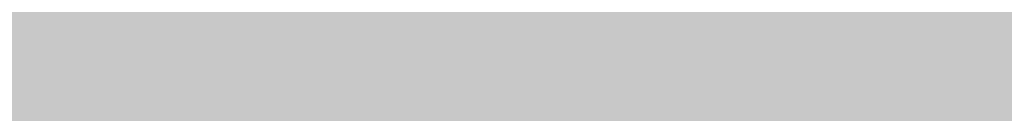
# Model space of a CAD drawing. Units: millimetres. Extents: x 0 to 2267, y 0 to 1823.
# Tile 52 of 256: x 1596.855 to 1600.369, y 1226.386 to 1226.718. Entities that reach past the tile are written whole.
import ezdxf

# ---------------------------------------------------------------- set-up
doc = ezdxf.new("R2010")
doc.units = ezdxf.units.MM
doc.header["$MEASUREMENT"] = 0
doc.layers.add('M-HATC', color=252, linetype='Continuous', lineweight=18)

msp = doc.modelspace()

# ---------------------------------------------------------------- hatches: boundary and pattern name
at = {"layer": 'M-HATC'}
h = msp.add_hatch(color=256, dxfattribs=at)
h.dxf.hatch_style = 1
h.paths.add_polyline_path([(2055.771, 1603.062), (1381.0868, 1603.062), (1381.0868, 1598.062), (2055.771, 1598.062)])
h.paths.add_polyline_path([(2055.771, 1598.062), (1381.0868, 1598.062), (1381.0868, 1593.062), (2055.771, 1593.062)])
h.paths.add_polyline_path([(2051.3074, 1536.7609), (1385.5504, 1536.7609), (1385.5504, 1526.7609), (1387.5504, 1526.7609), (1388.5366, 1525.0528), (1385.3319, 1521.2335), (1385.3319, 1521.2226), (2050.2542, 1522.7491), (2048.3212, 1525.0528), (2049.3074, 1526.7609), (2051.3074, 1526.7609)])
edge = h.paths.add_edge_path()
edge.add_arc((1847.5345, 1379.1492), 135, 222.603061, 222.890851, ccw=False)
edge.add_line((1748.1663, 1287.7656), (1683.0921, 1287.7656))
edge.add_arc((1583.7239, 1379.1492), 135, 317.109149, 317.396939, ccw=False)
edge.add_arc((1678.9686, 1290.6707), 5, 222.8909, 317.1091, ccw=False)
edge.add_arc((1774.2133, 1379.1492), 135, 222.603061, 222.890851, ccw=False)
edge.add_line((1674.8451, 1287.7656), (1609.7709, 1287.7656))
edge.add_arc((1510.4027, 1379.1492), 135, 317.109149, 317.396939, ccw=False)
edge.add_arc((1605.6474, 1290.6707), 5, 222.8909, 317.1091, ccw=False)
edge.add_arc((1700.8921, 1379.1492), 135, 222.603061, 222.890851, ccw=False)
edge.add_line((1601.5239, 1287.7656), (1536.4497, 1287.7656))
edge.add_arc((1437.0815, 1379.1492), 135, 317.109149, 317.396939, ccw=False)
edge.add_arc((1532.3262, 1290.6707), 5, 222.8909, 317.1091, ccw=False)
edge.add_arc((1627.5709, 1379.1492), 135, 222.603061, 222.890851, ccw=False)
edge.add_line((1528.2027, 1287.7656), (1505.9289, 1287.7656))
edge.add_spline(control_points=[(1505.9289, 1287.7656), (1504.2622, 1287.7656), (1504.2622, 1282.7656), (1505.9289, 1282.7656)], knot_values=[0, 0, 0, 0, 5, 5, 5, 5], degree=3, periodic=0)
edge.add_line((1505.9289, 1282.7656), (1930.9289, 1282.7656))
edge.add_spline(control_points=[(1930.9289, 1282.7656), (1932.5956, 1282.7656), (1932.5956, 1287.7656), (1930.9289, 1287.7656)], knot_values=[0, 0, 0, 0, 5, 5, 5, 5], degree=3, periodic=0)
edge.add_line((1930.9289, 1287.7656), (1903.0557, 1287.7656))
edge.add_arc((1803.6875, 1379.1492), 135, 317.109149, 317.396939, ccw=False)
edge.add_arc((1898.9322, 1290.6707), 5, 222.8909, 317.1091, ccw=False)
edge.add_arc((1994.1769, 1379.1492), 135, 222.603061, 222.890851, ccw=False)
edge.add_line((1894.8087, 1287.7656), (1829.7345, 1287.7656))
edge.add_arc((1730.3663, 1379.1492), 135, 317.109149, 317.396939, ccw=False)
edge.add_arc((1825.611, 1290.6707), 5, 222.8909, 317.1091, ccw=False)
edge.add_arc((1920.8557, 1379.1492), 135, 222.603061, 222.890851, ccw=False)
edge.add_line((1821.4875, 1287.7656), (1756.4133, 1287.7656))
edge.add_arc((1657.0451, 1379.1492), 135, 317.109149, 317.396939, ccw=False)
edge.add_arc((1752.2898, 1290.6707), 5, 222.8909, 317.1091, ccw=False)
edge = h.paths.add_edge_path()
edge.add_spline(control_points=[(1843.4289, 1227.2475), (1845.0956, 1227.2475), (1845.0956, 1232.2475), (1843.4289, 1232.2475)], knot_values=[0, 0, 0, 0, 5, 5, 5, 5], degree=3, periodic=0)
edge.add_line((1843.4289, 1232.2475), (1593.4289, 1232.2475))
edge.add_spline(control_points=[(1593.4289, 1232.2475), (1591.7622, 1232.2475), (1591.7622, 1227.2475), (1593.4289, 1227.2475)], knot_values=[0, 0, 0, 0, 5, 5, 5, 5], degree=3, periodic=0)
edge.add_line((1593.4289, 1227.2475), (1843.4289, 1227.2475))
h.paths.add_polyline_path([(1905.9289, 1127.4171), (1530.9289, 1127.4171, 0.414214), (1520.9289, 1117.4171), (1530.9289, 1117.4171), (1915.9289, 1117.4171, 0.414214)])
edge = h.paths.add_edge_path()
edge.add_arc((1397.0858, 1498.4078), 12.7299, 90.78215, 190.87871, ccw=False)
edge.add_line((1396.912, 1511.1365), (1428.0097, 1511.3488))
edge.add_line((1428.0097, 1511.3488), (1433.0097, 1511.3488))
edge.add_line((1433.0097, 1511.3488), (1434.439, 1511.3488))
edge.add_arc((1419.474, 1498.0804), 20, 41.561, 74.08211)
edge.add_line((1424.9592, 1517.3135), (1399.9351, 1517.2561))
edge.add_spline(control_points=[(1399.9307, 1517.2561), (1399.884, 1517.2131), (1399.8328, 1517.1689), (1399.7774, 1517.1236)], knot_values=[11.567499, 11.567499, 11.567499, 11.567499, 11.814249, 11.814249, 11.814249, 11.814249], degree=3, periodic=0)
edge.add_spline(control_points=[(1399.6328, 1517.0099), (1399.5831, 1516.9721), (1399.5307, 1516.9338), (1399.4759, 1516.8947)], knot_values=[11.167718, 11.167718, 11.167718, 11.167718, 11.365188, 11.365188, 11.365188, 11.365188], degree=3, periodic=0)
edge.add_spline(control_points=[(1399.3398, 1516.8001), (1399.1514, 1516.6719), (1398.9384, 1516.5377), (1398.704, 1516.3994)], knot_values=[10.376405, 10.376405, 10.376405, 10.376405, 11.00994, 11.00994, 11.00994, 11.00994], degree=3, periodic=0)
edge.add_spline(control_points=[(1398.6572, 1516.3719), (1398.5789, 1516.326), (1398.4983, 1516.2797), (1398.4155, 1516.2331)], knot_values=[10.125175, 10.125175, 10.125175, 10.125175, 10.334406, 10.334406, 10.334406, 10.334406], degree=3, periodic=0)
edge.add_spline(control_points=[(1398.2642, 1516.1487), (1398.196, 1516.1111), (1398.1263, 1516.0732), (1398.0555, 1516.0351)], knot_values=[9.832246, 9.832246, 9.832246, 9.832246, 9.999658, 9.999658, 9.999658, 9.999658], degree=3, periodic=0)
edge.add_spline(control_points=[(1397.9987, 1516.0048), (1397.7312, 1515.8621), (1397.446, 1515.7171), (1397.1466, 1515.5714)], knot_values=[9.161808, 9.161808, 9.161808, 9.161808, 9.787769, 9.787769, 9.787769, 9.787769], degree=3, periodic=0)
edge.add_spline(control_points=[(1397.1466, 1515.5714), (1396.8418, 1515.423), (1396.5222, 1515.274), (1396.1914, 1515.1262)], knot_values=[8.524455, 8.524455, 8.524455, 8.524455, 9.161808, 9.161808, 9.161808, 9.161808], degree=3, periodic=0)
edge.add_spline(control_points=[(1396.0777, 1515.0756), (1395.9854, 1515.0348), (1395.8922, 1514.994), (1395.7983, 1514.9534)], knot_values=[8.275193, 8.275193, 8.275193, 8.275193, 8.451726, 8.451726, 8.451726, 8.451726], degree=3, periodic=0)
edge.add_spline(control_points=[(1395.6018, 1514.8691), (1395.4997, 1514.8257), (1395.3968, 1514.7824), (1395.2932, 1514.7394)], knot_values=[7.962917, 7.962917, 7.962917, 7.962917, 8.152764, 8.152764, 8.152764, 8.152764], degree=3, periodic=0)
edge.add_spline(control_points=[(1395.2116, 1514.7057), (1394.8278, 1514.5475), (1394.4345, 1514.3929), (1394.0364, 1514.2442)], knot_values=[7.21254, 7.21254, 7.21254, 7.21254, 7.913148, 7.913148, 7.913148, 7.913148], degree=3, periodic=0)
edge.add_spline(control_points=[(1394.0364, 1514.2442), (1393.7076, 1514.1214), (1393.3754, 1514.0027), (1393.0427, 1513.8895)], knot_values=[6.633733, 6.633733, 6.633733, 6.633733, 7.21254, 7.21254, 7.21254, 7.21254], degree=3, periodic=0)
edge.add_spline(control_points=[(1392.8214, 1513.815), (1392.7198, 1513.7812), (1392.6181, 1513.7479), (1392.5166, 1513.7152)], knot_values=[6.328796, 6.328796, 6.328796, 6.328796, 6.505493, 6.505493, 6.505493, 6.505493], degree=3, periodic=0)
edge.add_spline(control_points=[(1392.5166, 1513.7152), (1392.3187, 1513.6515), (1392.1212, 1513.59), (1391.9244, 1513.531)], knot_values=[5.984605, 5.984605, 5.984605, 5.984605, 6.328796, 6.328796, 6.328796, 6.328796], degree=3, periodic=0)
edge.add_spline(control_points=[(1391.7915, 1513.4915), (1391.3122, 1513.3501), (1390.8384, 1513.2239), (1390.3784, 1513.1171)], knot_values=[5.066697, 5.066697, 5.066697, 5.066697, 5.907055, 5.907055, 5.907055, 5.907055], degree=3, periodic=0)
edge.add_spline(control_points=[(1390.3784, 1513.1171), (1390.1797, 1513.071), (1389.9836, 1513.0284), (1389.7907, 1512.9899)], knot_values=[4.70367, 4.70367, 4.70367, 4.70367, 5.066695, 5.066695, 5.066695, 5.066695], degree=3, periodic=0)
edge.add_spline(control_points=[(1389.422, 1512.9204), (1389.2459, 1512.8892), (1389.0729, 1512.8617), (1388.9036, 1512.8381)], knot_values=[4.130571, 4.130571, 4.130571, 4.130571, 4.469816, 4.469816, 4.469816, 4.469816], degree=3, periodic=0)
edge.add_spline(control_points=[(1388.9036, 1512.8381), (1388.591, 1512.7946), (1388.2911, 1512.7644), (1388.0071, 1512.7494)], knot_values=[3.504031, 3.504031, 3.504031, 3.504031, 4.130571, 4.130571, 4.130571, 4.130571], degree=3, periodic=0)
edge.add_spline(control_points=[(1387.9356, 1512.7459), (1387.8538, 1512.7423), (1387.7733, 1512.74), (1387.6944, 1512.739)], knot_values=[3.268866, 3.268866, 3.268866, 3.268866, 3.451164, 3.451164, 3.451164, 3.451164], degree=3, periodic=0)
edge.add_spline(control_points=[(1387.3351, 1512.7443), (1387.2076, 1512.7499), (1387.0847, 1512.7597), (1386.967, 1512.7739)], knot_values=[2.670686, 2.670686, 2.670686, 2.670686, 2.984, 2.984, 2.984, 2.984], degree=3, periodic=0)
edge.add_spline(control_points=[(1386.8327, 1512.7922), (1386.8209, 1512.7941), (1386.8092, 1512.7959), (1386.7975, 1512.7979)], knot_values=[2.516981, 2.516981, 2.516981, 2.516981, 2.549528, 2.549528, 2.549528, 2.549528], degree=3, periodic=0)
edge.add_spline(control_points=[(1386.4526, 1512.8735), (1386.4257, 1512.881), (1386.3993, 1512.889), (1386.3733, 1512.8972)], knot_values=[2.095869, 2.095869, 2.095869, 2.095869, 2.17941, 2.17941, 2.17941, 2.17941], degree=3, periodic=0)
edge.add_spline(control_points=[(1386.0691, 1513.0189), (1386.0634, 1513.0217), (1386.0577, 1513.0246), (1386.052, 1513.0275)], knot_values=[1.72453, 1.72453, 1.72453, 1.72453, 1.745933, 1.745933, 1.745933, 1.745933], degree=3, periodic=0)
edge.add_arc((1399.474, 1498.0804), 20, 131.82432, 180)
edge.add_arc((1630.3336, 1505.5484), 250.9708, 181.705176, 236.427975)
edge.add_arc((1605.3399, 1483.3044), 218.7822, 238.660829, 243.34961)
edge.add_arc((1647.0911, 1510.3592), 262.8986, 183.129836, 237.853442, ccw=False)
h.paths.add_polyline_path([(1406.5369, 1391.9644, 0.149382), (1491.5506, 1296.4418, -0.129517)], flags=17)
edge = h.paths.add_edge_path()
edge.add_arc((2037.3838, 1498.0804), 20, 0, 48.26587)
edge.add_spline(control_points=[(2050.6973, 1513.0052), (2050.6512, 1512.9847), (2050.6034, 1512.9655), (2050.5539, 1512.9477)], knot_values=[1.835652, 1.835652, 1.835652, 1.835652, 2.000781, 2.000781, 2.000781, 2.000781], degree=3, periodic=0)
edge.add_spline(control_points=[(2050.4616, 1512.9166), (2050.479, 1512.9221), (2050.4963, 1512.9277), (2050.5133, 1512.9335)], knot_values=[2.045477, 2.045477, 2.045477, 2.045477, 2.101389, 2.101389, 2.101389, 2.101389], degree=3, periodic=0)
edge.add_spline(control_points=[(2050.129, 1512.8342), (2050.1984, 1512.8473), (2050.2657, 1512.8623), (2050.3308, 1512.8792)], knot_values=[2.237629, 2.237629, 2.237629, 2.237629, 2.435841, 2.435841, 2.435841, 2.435841], degree=3, periodic=0)
edge.add_spline(control_points=[(2050.0946, 1512.8278), (2050.1061, 1512.8299), (2050.1176, 1512.832), (2050.129, 1512.8342)], knot_values=[2.435841, 2.435841, 2.435841, 2.435841, 2.468321, 2.468321, 2.468321, 2.468321], degree=3, periodic=0)
edge.add_spline(control_points=[(2049.7843, 1512.7851), (2049.8552, 1512.7922), (2049.9243, 1512.8008), (2049.9917, 1512.8109)], knot_values=[2.563852, 2.563852, 2.563852, 2.563852, 2.748541, 2.748541, 2.748541, 2.748541], degree=3, periodic=0)
edge.add_spline(control_points=[(2049.4052, 1512.7617), (2049.5364, 1512.7653), (2049.6629, 1512.773), (2049.7843, 1512.7851)], knot_values=[2.748541, 2.748541, 2.748541, 2.748541, 3.064882, 3.064882, 3.064882, 3.064882], degree=3, periodic=0)
edge.add_spline(control_points=[(2049.1698, 1512.7597), (2049.2336, 1512.7591), (2049.2965, 1512.7594), (2049.3584, 1512.7606)], knot_values=[3.102309, 3.102309, 3.102309, 3.102309, 3.2503, 3.2503, 3.2503, 3.2503], degree=3, periodic=0)
edge.add_spline(control_points=[(2048.8573, 1512.7691), (2048.9638, 1512.7638), (2049.068, 1512.7606), (2049.1698, 1512.7597)], knot_values=[3.2503, 3.2503, 3.2503, 3.2503, 3.486069, 3.486069, 3.486069, 3.486069], degree=3, periodic=0)
edge.add_spline(control_points=[(2048.6924, 1512.7789), (2048.3729, 1512.8009), (2048.0345, 1512.8411), (2047.6817, 1512.897)], knot_values=[3.606429, 3.606429, 3.606429, 3.606429, 4.2989, 4.2989, 4.2989, 4.2989], degree=3, periodic=0)
edge.add_spline(control_points=[(2047.6817, 1512.897), (2047.5458, 1512.9185), (2047.4077, 1512.9424), (2047.2678, 1512.9685)], knot_values=[4.2989, 4.2989, 4.2989, 4.2989, 4.565769, 4.565769, 4.565769, 4.565769], degree=3, periodic=0)
edge.add_spline(control_points=[(2047.2678, 1512.9685), (2047.1449, 1512.9914), (2047.0207, 1513.016), (2046.8951, 1513.0422)], knot_values=[4.565769, 4.565769, 4.565769, 4.565769, 4.799971, 4.799971, 4.799971, 4.799971], degree=3, periodic=0)
edge.add_spline(control_points=[(2046.8951, 1513.0422), (2046.5286, 1513.1188), (2046.1513, 1513.209), (2045.7676, 1513.3107)], knot_values=[4.799971, 4.799971, 4.799971, 4.799971, 5.483718, 5.483718, 5.483718, 5.483718], degree=3, periodic=0)
edge.add_spline(control_points=[(2045.7676, 1513.3107), (2045.3724, 1513.4154), (2044.9704, 1513.5322), (2044.5662, 1513.6588)], knot_values=[5.483718, 5.483718, 5.483718, 5.483718, 6.187866, 6.187866, 6.187866, 6.187866], degree=3, periodic=0)
edge.add_spline(control_points=[(2044.5662, 1513.6588), (2044.4149, 1513.7061), (2044.2633, 1513.7549), (2044.1116, 1513.8048)], knot_values=[6.187866, 6.187866, 6.187866, 6.187866, 6.451551, 6.451551, 6.451551, 6.451551], degree=3, periodic=0)
edge.add_spline(control_points=[(2044.1116, 1513.8048), (2043.9967, 1513.8427), (2043.8817, 1513.8813), (2043.7668, 1513.9205)], knot_values=[6.451551, 6.451551, 6.451551, 6.451551, 6.651434, 6.651434, 6.651434, 6.651434], degree=3, periodic=0)
edge.add_spline(control_points=[(2043.7668, 1513.9205), (2043.3716, 1514.0554), (2042.9774, 1514.1979), (2042.5886, 1514.3458)], knot_values=[6.651434, 6.651434, 6.651434, 6.651434, 7.338879, 7.338879, 7.338879, 7.338879], degree=3, periodic=0)
edge.add_spline(control_points=[(2042.5886, 1514.3458), (2042.1643, 1514.5071), (2041.7465, 1514.6749), (2041.3409, 1514.846)], knot_values=[7.338879, 7.338879, 7.338879, 7.338879, 8.089209, 8.089209, 8.089209, 8.089209], degree=3, periodic=0)
edge.add_spline(control_points=[(2041.3409, 1514.846), (2041.1028, 1514.9465), (2040.869, 1515.0481), (2040.6405, 1515.1502)], knot_values=[8.089209, 8.089209, 8.089209, 8.089209, 8.529587, 8.529587, 8.529587, 8.529587], degree=3, periodic=0)
edge.add_spline(control_points=[(2040.51, 1515.2089), (2040.0824, 1515.4022), (2039.6747, 1515.5971), (2039.295, 1515.7894)], knot_values=[8.613818, 8.613818, 8.613818, 8.613818, 9.44571, 9.44571, 9.44571, 9.44571], degree=3, periodic=0)
edge.add_spline(control_points=[(2039.295, 1515.7894), (2039.0618, 1515.9075), (2038.8391, 1516.0246), (2038.6288, 1516.1398)], knot_values=[9.44571, 9.44571, 9.44571, 9.44571, 9.956404, 9.956404, 9.956404, 9.956404], degree=3, periodic=0)
edge.add_spline(control_points=[(2038.6288, 1516.1398), (2038.5187, 1516.2001), (2038.4121, 1516.2598), (2038.309, 1516.3189)], knot_values=[9.956404, 9.956404, 9.956404, 9.956404, 10.223542, 10.223542, 10.223542, 10.223542], degree=3, periodic=0)
edge.add_spline(control_points=[(2038.309, 1516.3189), (2038.2138, 1516.3735), (2038.1216, 1516.4276), (2038.0328, 1516.481)], knot_values=[10.223542, 10.223542, 10.223542, 10.223542, 10.47051, 10.47051, 10.47051, 10.47051], degree=3, periodic=0)
edge.add_spline(control_points=[(2038.0328, 1516.481), (2037.7855, 1516.6296), (2037.5639, 1516.773), (2037.3722, 1516.909)], knot_values=[10.47051, 10.47051, 10.47051, 10.47051, 11.15767, 11.15767, 11.15767, 11.15767], degree=3, periodic=0)
edge.add_spline(control_points=[(2037.3722, 1516.909), (2037.2789, 1516.9752), (2037.1927, 1517.0396), (2037.1142, 1517.102)], knot_values=[11.15767, 11.15767, 11.15767, 11.15767, 11.49227, 11.49227, 11.49227, 11.49227], degree=3, periodic=0)
edge.add_spline(control_points=[(2036.8564, 1517.3259), (2036.9148, 1517.2692), (2036.9814, 1517.2103), (2037.0557, 1517.1492)], knot_values=[11.577341, 11.577341, 11.577341, 11.577341, 11.91035, 11.91035, 11.91035, 11.91035], degree=3, periodic=0)
edge.add_spline(control_points=[(2036.8074, 1517.3748), (2036.823, 1517.3587), (2036.8393, 1517.3424), (2036.8564, 1517.3259)], knot_values=[11.91035, 11.91035, 11.91035, 11.91035, 12.007402, 12.007402, 12.007402, 12.007402], degree=3, periodic=0)
edge.add_spline(control_points=[(2036.7017, 1517.494), (2036.7104, 1517.483), (2036.7196, 1517.4719), (2036.7291, 1517.4606)], knot_values=[12.184155, 12.184155, 12.184155, 12.184155, 12.255409, 12.255409, 12.255409, 12.255409], degree=3, periodic=0)
edge.add_spline(control_points=[(2036.6159, 1517.6205), (2036.62, 1517.613), (2036.6243, 1517.6055), (2036.6289, 1517.5979)], knot_values=[12.487913, 12.487913, 12.487913, 12.487913, 12.541035, 12.541035, 12.541035, 12.541035], degree=3, periodic=0)
edge.add_spline(control_points=[(2036.5635, 1517.786), (2036.5637, 1517.7794), (2036.5642, 1517.7726), (2036.565, 1517.7658)], knot_values=[12.911761, 12.911761, 12.911761, 12.911761, 12.968286, 12.968286, 12.968286, 12.968286], degree=3, periodic=0)
edge.add_spline(control_points=[(2036.6166, 1517.9304), (2036.6125, 1517.9259), (2036.6086, 1517.9212), (2036.6049, 1517.9165)], knot_values=[13.382527, 13.382527, 13.382527, 13.382527, 13.433791, 13.433791, 13.433791, 13.433791], degree=3, periodic=0)
edge.add_spline(control_points=[(2036.749, 1518.017), (2036.7361, 1518.0116), (2036.7239, 1518.006), (2036.7124, 1518.0002)], knot_values=[13.726299, 13.726299, 13.726299, 13.726299, 13.809928, 13.809928, 13.809928, 13.809928], degree=3, periodic=0)
edge.add_spline(control_points=[(2036.8604, 1518.0528), (2036.8386, 1518.0474), (2036.8181, 1518.0416), (2036.7988, 1518.0353)], knot_values=[13.910887, 13.910887, 13.910887, 13.910887, 14.02153, 14.02153, 14.02153, 14.02153], degree=3, periodic=0)
edge.add_line((2036.9639, 1518.0804), (2032.3838, 1518.0804))
edge.add_line((2032.3838, 1518.0804), (2027.3838, 1518.0804))
edge.add_line((2027.3838, 1518.0804), (2022.3838, 1518.0804))
edge.add_line((2022.3838, 1518.0804), (2017.3838, 1518.0804))
edge.add_arc((2017.3838, 1498.0804), 20, 90, 138.439)
edge.add_line((2002.4188, 1511.3488), (2003.8481, 1511.3488))
edge.add_line((2003.8481, 1511.3488), (2008.8481, 1511.3488))
edge.add_line((2008.8481, 1511.3488), (2039.772, 1511.1377))
edge.add_arc((2039.772, 1498.4078), 12.7299, -10.87871, 90, ccw=False)
edge.add_arc((1789.7668, 1510.3592), 262.8986, 302.146558, 356.870164, ccw=False)
edge.add_arc((1831.5179, 1483.3044), 218.7822, 296.65039, 301.339171)
edge.add_arc((1806.5242, 1505.5484), 250.9708, 303.572025, 358.294824)
h.paths.add_polyline_path([(2030.321, 1391.9644, -0.129517), (1945.3072, 1296.4418, 0.149382)], flags=17)
edge = h.paths.add_edge_path()
edge.add_spline(control_points=[(2037.2464, 1518.0821), (2037.2898, 1518.081), (2037.3355, 1518.0804), (2037.3838, 1518.0804)], knot_values=[0.000012, 0.000012, 0.000012, 0.000012, 0.144754, 0.144754, 0.144754, 0.144754], degree=3, periodic=0)
edge.add_line((2037.3357, 1518.0804), (2037.0096, 1518.0804))
edge.add_spline(control_points=[(2037.0096, 1518.0804), (2036.9822, 1518.0768), (2036.956, 1518.0727), (2036.9312, 1518.0681)], knot_values=[14.13465, 14.13465, 14.13465, 14.13465, 14.247197, 14.247197, 14.247197, 14.247197], degree=3, periodic=0)
edge.add_spline(control_points=[(2036.9312, 1518.0681), (2036.9276, 1518.0674), (2036.9241, 1518.0667), (2036.9205, 1518.0661)], knot_values=[14.118315, 14.118315, 14.118315, 14.118315, 14.13465, 14.13465, 14.13465, 14.13465], degree=3, periodic=0)
edge.add_spline(control_points=[(2036.9205, 1518.0661), (2036.9118, 1518.0644), (2036.9032, 1518.0626), (2036.8948, 1518.0608)], knot_values=[14.078086, 14.078086, 14.078086, 14.078086, 14.118315, 14.118315, 14.118315, 14.118315], degree=3, periodic=0)
edge.add_spline(control_points=[(2036.8948, 1518.0608), (2036.883, 1518.0583), (2036.8716, 1518.0556), (2036.8604, 1518.0528)], knot_values=[14.02153, 14.02153, 14.02153, 14.02153, 14.078086, 14.078086, 14.078086, 14.078086], degree=3, periodic=0)
edge.add_spline(control_points=[(2036.8604, 1518.0528), (2036.8386, 1518.0474), (2036.8181, 1518.0416), (2036.7988, 1518.0353)], knot_values=[13.910887, 13.910887, 13.910887, 13.910887, 14.02153, 14.02153, 14.02153, 14.02153], degree=3, periodic=0)
edge.add_spline(control_points=[(2036.7988, 1518.0353), (2036.7981, 1518.035), (2036.7974, 1518.0348), (2036.7967, 1518.0346)], knot_values=[13.906906, 13.906906, 13.906906, 13.906906, 13.910887, 13.910887, 13.910887, 13.910887], degree=3, periodic=0)
edge.add_spline(control_points=[(2036.7967, 1518.0346), (2036.7882, 1518.0318), (2036.7799, 1518.0289), (2036.7719, 1518.0259)], knot_values=[13.857826, 13.857826, 13.857826, 13.857826, 13.906906, 13.906906, 13.906906, 13.906906], degree=3, periodic=0)
edge.add_spline(control_points=[(2036.7719, 1518.0259), (2036.764, 1518.023), (2036.7564, 1518.02), (2036.749, 1518.017)], knot_values=[13.809928, 13.809928, 13.809928, 13.809928, 13.857826, 13.857826, 13.857826, 13.857826], degree=3, periodic=0)
edge.add_spline(control_points=[(2036.749, 1518.017), (2036.7361, 1518.0116), (2036.7239, 1518.006), (2036.7124, 1518.0002)], knot_values=[13.726299, 13.726299, 13.726299, 13.726299, 13.809928, 13.809928, 13.809928, 13.809928], degree=3, periodic=0)
edge.add_spline(control_points=[(2036.7124, 1518.0002), (2036.7121, 1518), (2036.7118, 1517.9999), (2036.7115, 1517.9997)], knot_values=[13.723993, 13.723993, 13.723993, 13.723993, 13.726299, 13.726299, 13.726299, 13.726299], degree=3, periodic=0)
edge.add_spline(control_points=[(2036.7115, 1517.9997), (2036.7063, 1517.9971), (2036.7013, 1517.9944), (2036.6965, 1517.9917)], knot_values=[13.686536, 13.686536, 13.686536, 13.686536, 13.723993, 13.723993, 13.723993, 13.723993], degree=3, periodic=0)
edge.add_spline(control_points=[(2036.6965, 1517.9917), (2036.6919, 1517.9891), (2036.6874, 1517.9865), (2036.6831, 1517.9839)], knot_values=[13.651251, 13.651251, 13.651251, 13.651251, 13.686536, 13.686536, 13.686536, 13.686536], degree=3, periodic=0)
edge.add_spline(control_points=[(2036.6831, 1517.9839), (2036.6764, 1517.9798), (2036.67, 1517.9757), (2036.6639, 1517.9714)], knot_values=[13.596804, 13.596804, 13.596804, 13.596804, 13.651251, 13.651251, 13.651251, 13.651251], degree=3, periodic=0)
edge.add_spline(control_points=[(2036.6639, 1517.9714), (2036.6636, 1517.9712), (2036.6633, 1517.9709), (2036.6629, 1517.9707)], knot_values=[13.593956, 13.593956, 13.593956, 13.593956, 13.596804, 13.596804, 13.596804, 13.596804], degree=3, periodic=0)
edge.add_spline(control_points=[(2036.6629, 1517.9707), (2036.6603, 1517.9689), (2036.6577, 1517.967), (2036.6552, 1517.9651)], knot_values=[13.570322, 13.570322, 13.570322, 13.570322, 13.593956, 13.593956, 13.593956, 13.593956], degree=3, periodic=0)
edge.add_spline(control_points=[(2036.6552, 1517.9651), (2036.6525, 1517.9631), (2036.6499, 1517.9611), (2036.6474, 1517.9591)], knot_values=[13.545477, 13.545477, 13.545477, 13.545477, 13.570322, 13.570322, 13.570322, 13.570322], degree=3, periodic=0)
edge.add_spline(control_points=[(2036.6474, 1517.9591), (2036.6472, 1517.9589), (2036.6471, 1517.9588), (2036.6469, 1517.9587)], knot_values=[13.543931, 13.543931, 13.543931, 13.543931, 13.545477, 13.545477, 13.545477, 13.545477], degree=3, periodic=0)
edge.add_spline(control_points=[(2036.6469, 1517.9587), (2036.6412, 1517.9541), (2036.6358, 1517.9494), (2036.6307, 1517.9447)], knot_values=[13.488237, 13.488237, 13.488237, 13.488237, 13.543931, 13.543931, 13.543931, 13.543931], degree=3, periodic=0)
edge.add_spline(control_points=[(2036.6307, 1517.9447), (2036.6282, 1517.9423), (2036.6257, 1517.9399), (2036.6233, 1517.9374)], knot_values=[13.460307, 13.460307, 13.460307, 13.460307, 13.488237, 13.488237, 13.488237, 13.488237], degree=3, periodic=0)
edge.add_spline(control_points=[(2036.6233, 1517.9374), (2036.6215, 1517.9356), (2036.6198, 1517.9338), (2036.6181, 1517.932)], knot_values=[13.439712, 13.439712, 13.439712, 13.439712, 13.460307, 13.460307, 13.460307, 13.460307], degree=3, periodic=0)
edge.add_spline(control_points=[(2036.6181, 1517.932), (2036.6176, 1517.9315), (2036.6171, 1517.9309), (2036.6166, 1517.9304)], knot_values=[13.433791, 13.433791, 13.433791, 13.433791, 13.439712, 13.439712, 13.439712, 13.439712], degree=3, periodic=0)
edge.add_spline(control_points=[(2036.6166, 1517.9304), (2036.6125, 1517.9259), (2036.6086, 1517.9212), (2036.6049, 1517.9165)], knot_values=[13.382527, 13.382527, 13.382527, 13.382527, 13.433791, 13.433791, 13.433791, 13.433791], degree=3, periodic=0)
edge.add_spline(control_points=[(2036.6049, 1517.9165), (2036.6026, 1517.9135), (2036.6004, 1517.9104), (2036.5982, 1517.9074)], knot_values=[13.350017, 13.350017, 13.350017, 13.350017, 13.382527, 13.382527, 13.382527, 13.382527], degree=3, periodic=0)
edge.add_spline(control_points=[(2036.5982, 1517.9074), (2036.5972, 1517.9059), (2036.5962, 1517.9043), (2036.5952, 1517.9028)], knot_values=[13.333922, 13.333922, 13.333922, 13.333922, 13.350017, 13.350017, 13.350017, 13.350017], degree=3, periodic=0)
edge.add_spline(control_points=[(2036.5952, 1517.9028), (2036.5945, 1517.9018), (2036.5939, 1517.9009), (2036.5933, 1517.8999)], knot_values=[13.323828, 13.323828, 13.323828, 13.323828, 13.333922, 13.333922, 13.333922, 13.333922], degree=3, periodic=0)
edge.add_spline(control_points=[(2036.5933, 1517.8999), (2036.5905, 1517.8955), (2036.5879, 1517.8909), (2036.5855, 1517.8864)], knot_values=[13.277545, 13.277545, 13.277545, 13.277545, 13.323828, 13.323828, 13.323828, 13.323828], degree=3, periodic=0)
edge.add_spline(control_points=[(2036.5855, 1517.8864), (2036.5836, 1517.8827), (2036.5817, 1517.8789), (2036.5801, 1517.8751)], knot_values=[13.240119, 13.240119, 13.240119, 13.240119, 13.277545, 13.277545, 13.277545, 13.277545], degree=3, periodic=0)
edge.add_spline(control_points=[(2036.5801, 1517.8751), (2036.5795, 1517.8739), (2036.579, 1517.8727), (2036.5785, 1517.8715)], knot_values=[13.228211, 13.228211, 13.228211, 13.228211, 13.240119, 13.240119, 13.240119, 13.240119], degree=3, periodic=0)
edge.add_spline(control_points=[(2036.5785, 1517.8715), (2036.578, 1517.8702), (2036.5774, 1517.869), (2036.5769, 1517.8677)], knot_values=[13.215717, 13.215717, 13.215717, 13.215717, 13.228211, 13.228211, 13.228211, 13.228211], degree=3, periodic=0)
edge.add_spline(control_points=[(2036.5769, 1517.8677), (2036.5755, 1517.864), (2036.5741, 1517.8603), (2036.5729, 1517.8565)], knot_values=[13.179847, 13.179847, 13.179847, 13.179847, 13.215717, 13.215717, 13.215717, 13.215717], degree=3, periodic=0)
edge.add_spline(control_points=[(2036.5729, 1517.8565), (2036.5713, 1517.8515), (2036.5699, 1517.8464), (2036.5687, 1517.8413)], knot_values=[13.132017, 13.132017, 13.132017, 13.132017, 13.179847, 13.179847, 13.179847, 13.179847], degree=3, periodic=0)
edge.add_spline(control_points=[(2036.5687, 1517.8413), (2036.5684, 1517.8402), (2036.5682, 1517.8392), (2036.568, 1517.8382)], knot_values=[13.122482, 13.122482, 13.122482, 13.122482, 13.132017, 13.132017, 13.132017, 13.132017], degree=3, periodic=0)
edge.add_spline(control_points=[(2036.568, 1517.8382), (2036.5676, 1517.8363), (2036.5672, 1517.8345), (2036.5669, 1517.8327)], knot_values=[13.105592, 13.105592, 13.105592, 13.105592, 13.122482, 13.122482, 13.122482, 13.122482], degree=3, periodic=0)
edge.add_spline(control_points=[(2036.5669, 1517.8327), (2036.5662, 1517.8292), (2036.5657, 1517.8257), (2036.5652, 1517.8222)], knot_values=[13.074063, 13.074063, 13.074063, 13.074063, 13.105592, 13.105592, 13.105592, 13.105592], degree=3, periodic=0)
edge.add_spline(control_points=[(2036.5652, 1517.8222), (2036.5652, 1517.8222), (2036.5652, 1517.8222), (2036.5652, 1517.8222)], knot_values=[13.074043, 13.074043, 13.074043, 13.074043, 13.074063, 13.074063, 13.074063, 13.074063], degree=3, periodic=0)
edge.add_spline(control_points=[(2036.5652, 1517.8222), (2036.5644, 1517.8164), (2036.5639, 1517.8106), (2036.5636, 1517.8046)], knot_values=[13.021884, 13.021884, 13.021884, 13.021884, 13.074043, 13.074043, 13.074043, 13.074043], degree=3, periodic=0)
edge.add_spline(control_points=[(2036.5636, 1517.8046), (2036.5636, 1517.804), (2036.5636, 1517.8034), (2036.5635, 1517.8028)], knot_values=[13.01674, 13.01674, 13.01674, 13.01674, 13.021884, 13.021884, 13.021884, 13.021884], degree=3, periodic=0)
edge.add_spline(control_points=[(2036.5635, 1517.8028), (2036.5634, 1517.8005), (2036.5634, 1517.7982), (2036.5634, 1517.7958)], knot_values=[12.996438, 12.996438, 12.996438, 12.996438, 13.01674, 13.01674, 13.01674, 13.01674], degree=3, periodic=0)
edge.add_spline(control_points=[(2036.5634, 1517.7958), (2036.5633, 1517.7926), (2036.5634, 1517.7893), (2036.5635, 1517.786)], knot_values=[12.968286, 12.968286, 12.968286, 12.968286, 12.996438, 12.996438, 12.996438, 12.996438], degree=3, periodic=0)
edge.add_spline(control_points=[(2036.5635, 1517.786), (2036.5637, 1517.7794), (2036.5642, 1517.7726), (2036.565, 1517.7658)], knot_values=[12.911761, 12.911761, 12.911761, 12.911761, 12.968286, 12.968286, 12.968286, 12.968286], degree=3, periodic=0)
edge.add_spline(control_points=[(2036.565, 1517.7658), (2036.565, 1517.7657), (2036.565, 1517.7656), (2036.565, 1517.7656)], knot_values=[12.911017, 12.911017, 12.911017, 12.911017, 12.911761, 12.911761, 12.911761, 12.911761], degree=3, periodic=0)
edge.add_spline(control_points=[(2036.565, 1517.7656), (2036.5654, 1517.7625), (2036.5658, 1517.7593), (2036.5663, 1517.7562)], knot_values=[12.88528, 12.88528, 12.88528, 12.88528, 12.911017, 12.911017, 12.911017, 12.911017], degree=3, periodic=0)
edge.add_spline(control_points=[(2036.5663, 1517.7562), (2036.5667, 1517.7534), (2036.5672, 1517.7506), (2036.5677, 1517.7478)], knot_values=[12.862519, 12.862519, 12.862519, 12.862519, 12.88528, 12.88528, 12.88528, 12.88528], degree=3, periodic=0)
edge.add_spline(control_points=[(2036.5677, 1517.7478), (2036.5678, 1517.7474), (2036.5679, 1517.7469), (2036.568, 1517.7465)], knot_values=[12.858885, 12.858885, 12.858885, 12.858885, 12.862519, 12.862519, 12.862519, 12.862519], degree=3, periodic=0)
edge.add_spline(control_points=[(2036.568, 1517.7465), (2036.5692, 1517.7399), (2036.5707, 1517.7332), (2036.5724, 1517.7264)], knot_values=[12.8053, 12.8053, 12.8053, 12.8053, 12.858885, 12.858885, 12.858885, 12.858885], degree=3, periodic=0)
edge.add_spline(control_points=[(2036.5724, 1517.7264), (2036.5734, 1517.7226), (2036.5745, 1517.7187), (2036.5756, 1517.7149)], knot_values=[12.775176, 12.775176, 12.775176, 12.775176, 12.8053, 12.8053, 12.8053, 12.8053], degree=3, periodic=0)
edge.add_spline(control_points=[(2036.5756, 1517.7149), (2036.5763, 1517.7125), (2036.577, 1517.7102), (2036.5778, 1517.7078)], knot_values=[12.756759, 12.756759, 12.756759, 12.756759, 12.775176, 12.775176, 12.775176, 12.775176], degree=3, periodic=0)
edge.add_spline(control_points=[(2036.5778, 1517.7078), (2036.5781, 1517.7067), (2036.5784, 1517.7057), (2036.5787, 1517.7047)], knot_values=[12.748742, 12.748742, 12.748742, 12.748742, 12.756759, 12.756759, 12.756759, 12.756759], degree=3, periodic=0)
edge.add_spline(control_points=[(2036.5787, 1517.7047), (2036.5808, 1517.6983), (2036.5831, 1517.6919), (2036.5856, 1517.6854)], knot_values=[12.69959, 12.69959, 12.69959, 12.69959, 12.748742, 12.748742, 12.748742, 12.748742], degree=3, periodic=0)
edge.add_spline(control_points=[(2036.5856, 1517.6854), (2036.5876, 1517.68), (2036.5898, 1517.6746), (2036.5921, 1517.6692)], knot_values=[12.659038, 12.659038, 12.659038, 12.659038, 12.69959, 12.69959, 12.69959, 12.69959], degree=3, periodic=0)
edge.add_spline(control_points=[(2036.5921, 1517.6692), (2036.594, 1517.6648), (2036.5959, 1517.6605), (2036.5979, 1517.6561)], knot_values=[12.626806, 12.626806, 12.626806, 12.626806, 12.659038, 12.659038, 12.659038, 12.659038], degree=3, periodic=0)
edge.add_spline(control_points=[(2036.5979, 1517.6561), (2036.5984, 1517.6551), (2036.5989, 1517.6541), (2036.5993, 1517.6531)], knot_values=[12.619394, 12.619394, 12.619394, 12.619394, 12.626806, 12.626806, 12.626806, 12.626806], degree=3, periodic=0)
edge.add_spline(control_points=[(2036.5993, 1517.6531), (2036.6043, 1517.6424), (2036.6099, 1517.6315), (2036.6159, 1517.6205)], knot_values=[12.541039, 12.541039, 12.541039, 12.541039, 12.619394, 12.619394, 12.619394, 12.619394], degree=3, periodic=0)
edge.add_spline(control_points=[(2036.6159, 1517.6205), (2036.6159, 1517.6205), (2036.6159, 1517.6205), (2036.6159, 1517.6205)], knot_values=[12.541035, 12.541035, 12.541035, 12.541035, 12.541039, 12.541039, 12.541039, 12.541039], degree=3, periodic=0)
edge.add_spline(control_points=[(2036.6159, 1517.6205), (2036.62, 1517.613), (2036.6243, 1517.6055), (2036.6289, 1517.5979)], knot_values=[12.487913, 12.487913, 12.487913, 12.487913, 12.541035, 12.541035, 12.541035, 12.541035], degree=3, periodic=0)
edge.add_spline(control_points=[(2036.6289, 1517.5979), (2036.6326, 1517.5916), (2036.6365, 1517.5853), (2036.6406, 1517.5789)], knot_values=[12.443982, 12.443982, 12.443982, 12.443982, 12.487913, 12.487913, 12.487913, 12.487913], degree=3, periodic=0)
edge.add_spline(control_points=[(2036.6406, 1517.5789), (2036.6414, 1517.5776), (2036.6423, 1517.5763), (2036.6431, 1517.5749)], knot_values=[12.434996, 12.434996, 12.434996, 12.434996, 12.443982, 12.443982, 12.443982, 12.443982], degree=3, periodic=0)
edge.add_spline(control_points=[(2036.6431, 1517.5749), (2036.6531, 1517.5596), (2036.6639, 1517.5439), (2036.6756, 1517.528)], knot_values=[12.329647, 12.329647, 12.329647, 12.329647, 12.434996, 12.434996, 12.434996, 12.434996], degree=3, periodic=0)
edge.add_spline(control_points=[(2036.6756, 1517.528), (2036.6839, 1517.5168), (2036.6925, 1517.5055), (2036.7017, 1517.494)], knot_values=[12.255409, 12.255409, 12.255409, 12.255409, 12.329647, 12.329647, 12.329647, 12.329647], degree=3, periodic=0)
edge.add_spline(control_points=[(2036.7017, 1517.494), (2036.7104, 1517.483), (2036.7196, 1517.4719), (2036.7291, 1517.4606)], knot_values=[12.184155, 12.184155, 12.184155, 12.184155, 12.255409, 12.255409, 12.255409, 12.255409], degree=3, periodic=0)
edge.add_spline(control_points=[(2036.7291, 1517.4606), (2036.7436, 1517.4435), (2036.759, 1517.4262), (2036.7753, 1517.4085)], knot_values=[12.075961, 12.075961, 12.075961, 12.075961, 12.184155, 12.184155, 12.184155, 12.184155], degree=3, periodic=0)
edge.add_spline(control_points=[(2036.7753, 1517.4085), (2036.7763, 1517.4075), (2036.7773, 1517.4064), (2036.7783, 1517.4054)], knot_values=[12.069502, 12.069502, 12.069502, 12.069502, 12.075961, 12.075961, 12.075961, 12.075961], degree=3, periodic=0)
edge.add_spline(control_points=[(2036.7783, 1517.4054), (2036.7877, 1517.3953), (2036.7974, 1517.385), (2036.8074, 1517.3748)], knot_values=[12.007402, 12.007402, 12.007402, 12.007402, 12.069502, 12.069502, 12.069502, 12.069502], degree=3, periodic=0)
edge.add_spline(control_points=[(2036.8074, 1517.3748), (2036.823, 1517.3587), (2036.8393, 1517.3424), (2036.8564, 1517.3259)], knot_values=[11.91035, 11.91035, 11.91035, 11.91035, 12.007402, 12.007402, 12.007402, 12.007402], degree=3, periodic=0)
edge.add_spline(control_points=[(2036.8564, 1517.3259), (2036.9148, 1517.2692), (2036.9814, 1517.2103), (2037.0557, 1517.1492)], knot_values=[11.577341, 11.577341, 11.577341, 11.577341, 11.91035, 11.91035, 11.91035, 11.91035], degree=3, periodic=0)
edge.add_spline(control_points=[(2037.0557, 1517.1492), (2037.0747, 1517.1336), (2037.0942, 1517.1179), (2037.1142, 1517.102)], knot_values=[11.49227, 11.49227, 11.49227, 11.49227, 11.577341, 11.577341, 11.577341, 11.577341], degree=3, periodic=0)
edge.add_spline(control_points=[(2037.1142, 1517.102), (2037.1927, 1517.0396), (2037.2789, 1516.9752), (2037.3722, 1516.909)], knot_values=[11.15767, 11.15767, 11.15767, 11.15767, 11.49227, 11.49227, 11.49227, 11.49227], degree=3, periodic=0)
edge.add_spline(control_points=[(2037.3722, 1516.909), (2037.5639, 1516.773), (2037.7855, 1516.6296), (2038.0328, 1516.481)], knot_values=[10.47051, 10.47051, 10.47051, 10.47051, 11.15767, 11.15767, 11.15767, 11.15767], degree=3, periodic=0)
edge.add_spline(control_points=[(2038.0328, 1516.481), (2038.1216, 1516.4276), (2038.2138, 1516.3735), (2038.309, 1516.3189)], knot_values=[10.223542, 10.223542, 10.223542, 10.223542, 10.47051, 10.47051, 10.47051, 10.47051], degree=3, periodic=0)
edge.add_spline(control_points=[(2038.309, 1516.3189), (2038.4121, 1516.2598), (2038.5187, 1516.2001), (2038.6288, 1516.1398)], knot_values=[9.956404, 9.956404, 9.956404, 9.956404, 10.223542, 10.223542, 10.223542, 10.223542], degree=3, periodic=0)
edge.add_spline(control_points=[(2038.6288, 1516.1398), (2038.8391, 1516.0246), (2039.0618, 1515.9075), (2039.295, 1515.7894)], knot_values=[9.44571, 9.44571, 9.44571, 9.44571, 9.956404, 9.956404, 9.956404, 9.956404], degree=3, periodic=0)
edge.add_spline(control_points=[(2039.295, 1515.7894), (2039.6747, 1515.5971), (2040.0824, 1515.4022), (2040.51, 1515.2089)], knot_values=[8.613818, 8.613818, 8.613818, 8.613818, 9.44571, 9.44571, 9.44571, 9.44571], degree=3, periodic=0)
edge.add_spline(control_points=[(2040.51, 1515.2089), (2040.5533, 1515.1893), (2040.5968, 1515.1697), (2040.6405, 1515.1502)], knot_values=[8.529587, 8.529587, 8.529587, 8.529587, 8.613818, 8.613818, 8.613818, 8.613818], degree=3, periodic=0)
edge.add_spline(control_points=[(2040.6405, 1515.1502), (2040.869, 1515.0481), (2041.1028, 1514.9465), (2041.3409, 1514.846)], knot_values=[8.089209, 8.089209, 8.089209, 8.089209, 8.529587, 8.529587, 8.529587, 8.529587], degree=3, periodic=0)
edge.add_spline(control_points=[(2041.3409, 1514.846), (2041.7465, 1514.6749), (2042.1643, 1514.5071), (2042.5886, 1514.3458)], knot_values=[7.338879, 7.338879, 7.338879, 7.338879, 8.089209, 8.089209, 8.089209, 8.089209], degree=3, periodic=0)
edge.add_spline(control_points=[(2042.5886, 1514.3458), (2042.9774, 1514.1979), (2043.3716, 1514.0554), (2043.7668, 1513.9205)], knot_values=[6.651434, 6.651434, 6.651434, 6.651434, 7.338879, 7.338879, 7.338879, 7.338879], degree=3, periodic=0)
edge.add_spline(control_points=[(2043.7668, 1513.9205), (2043.8817, 1513.8813), (2043.9967, 1513.8427), (2044.1116, 1513.8048)], knot_values=[6.451551, 6.451551, 6.451551, 6.451551, 6.651434, 6.651434, 6.651434, 6.651434], degree=3, periodic=0)
edge.add_spline(control_points=[(2044.1116, 1513.8048), (2044.2633, 1513.7549), (2044.4149, 1513.7061), (2044.5662, 1513.6588)], knot_values=[6.187866, 6.187866, 6.187866, 6.187866, 6.451551, 6.451551, 6.451551, 6.451551], degree=3, periodic=0)
edge.add_spline(control_points=[(2044.5662, 1513.6588), (2044.9704, 1513.5322), (2045.3724, 1513.4154), (2045.7676, 1513.3107)], knot_values=[5.483718, 5.483718, 5.483718, 5.483718, 6.187866, 6.187866, 6.187866, 6.187866], degree=3, periodic=0)
edge.add_spline(control_points=[(2045.7676, 1513.3107), (2046.1513, 1513.209), (2046.5286, 1513.1188), (2046.8951, 1513.0422)], knot_values=[4.799971, 4.799971, 4.799971, 4.799971, 5.483718, 5.483718, 5.483718, 5.483718], degree=3, periodic=0)
edge.add_spline(control_points=[(2046.8951, 1513.0422), (2047.0207, 1513.016), (2047.1449, 1512.9914), (2047.2678, 1512.9685)], knot_values=[4.565769, 4.565769, 4.565769, 4.565769, 4.799971, 4.799971, 4.799971, 4.799971], degree=3, periodic=0)
edge.add_spline(control_points=[(2047.2678, 1512.9685), (2047.4077, 1512.9424), (2047.5458, 1512.9185), (2047.6817, 1512.897)], knot_values=[4.2989, 4.2989, 4.2989, 4.2989, 4.565769, 4.565769, 4.565769, 4.565769], degree=3, periodic=0)
edge.add_spline(control_points=[(2047.6817, 1512.897), (2048.0345, 1512.8411), (2048.3729, 1512.8009), (2048.6924, 1512.7789)], knot_values=[3.606429, 3.606429, 3.606429, 3.606429, 4.2989, 4.2989, 4.2989, 4.2989], degree=3, periodic=0)
edge.add_spline(control_points=[(2048.6924, 1512.7789), (2048.7479, 1512.7751), (2048.8029, 1512.7718), (2048.8573, 1512.7691)], knot_values=[3.486069, 3.486069, 3.486069, 3.486069, 3.606429, 3.606429, 3.606429, 3.606429], degree=3, periodic=0)
edge.add_spline(control_points=[(2048.8573, 1512.7691), (2048.9638, 1512.7638), (2049.068, 1512.7606), (2049.1698, 1512.7597)], knot_values=[3.2503, 3.2503, 3.2503, 3.2503, 3.486069, 3.486069, 3.486069, 3.486069], degree=3, periodic=0)
edge.add_spline(control_points=[(2049.1698, 1512.7597), (2049.2336, 1512.7591), (2049.2965, 1512.7594), (2049.3584, 1512.7606)], knot_values=[3.102309, 3.102309, 3.102309, 3.102309, 3.2503, 3.2503, 3.2503, 3.2503], degree=3, periodic=0)
edge.add_spline(control_points=[(2049.3584, 1512.7606), (2049.3741, 1512.7609), (2049.3897, 1512.7613), (2049.4052, 1512.7617)], knot_values=[3.064882, 3.064882, 3.064882, 3.064882, 3.102309, 3.102309, 3.102309, 3.102309], degree=3, periodic=0)
edge.add_spline(control_points=[(2049.4052, 1512.7617), (2049.5364, 1512.7653), (2049.6629, 1512.773), (2049.7843, 1512.7851)], knot_values=[2.748541, 2.748541, 2.748541, 2.748541, 3.064882, 3.064882, 3.064882, 3.064882], degree=3, periodic=0)
edge.add_spline(control_points=[(2049.7843, 1512.7851), (2049.8552, 1512.7922), (2049.9243, 1512.8008), (2049.9917, 1512.8109)], knot_values=[2.563852, 2.563852, 2.563852, 2.563852, 2.748541, 2.748541, 2.748541, 2.748541], degree=3, periodic=0)
edge.add_spline(control_points=[(2049.9917, 1512.8109), (2050.0265, 1512.8161), (2050.0608, 1512.8218), (2050.0946, 1512.8278)], knot_values=[2.468321, 2.468321, 2.468321, 2.468321, 2.563852, 2.563852, 2.563852, 2.563852], degree=3, periodic=0)
edge.add_spline(control_points=[(2050.0946, 1512.8278), (2050.1061, 1512.8299), (2050.1176, 1512.832), (2050.129, 1512.8342)], knot_values=[2.435841, 2.435841, 2.435841, 2.435841, 2.468321, 2.468321, 2.468321, 2.468321], degree=3, periodic=0)
edge.add_spline(control_points=[(2050.129, 1512.8342), (2050.1984, 1512.8473), (2050.2657, 1512.8623), (2050.3308, 1512.8792)], knot_values=[2.237629, 2.237629, 2.237629, 2.237629, 2.435841, 2.435841, 2.435841, 2.435841], degree=3, periodic=0)
edge.add_spline(control_points=[(2050.3308, 1512.8792), (2050.3754, 1512.8908), (2050.4191, 1512.9032), (2050.4616, 1512.9166)], knot_values=[2.101389, 2.101389, 2.101389, 2.101389, 2.237629, 2.237629, 2.237629, 2.237629], degree=3, periodic=0)
edge.add_spline(control_points=[(2050.4616, 1512.9166), (2050.479, 1512.9221), (2050.4963, 1512.9277), (2050.5133, 1512.9335)], knot_values=[2.045477, 2.045477, 2.045477, 2.045477, 2.101389, 2.101389, 2.101389, 2.101389], degree=3, periodic=0)
edge.add_spline(control_points=[(2050.5133, 1512.9335), (2050.527, 1512.9382), (2050.5405, 1512.9429), (2050.5539, 1512.9477)], knot_values=[2.000781, 2.000781, 2.000781, 2.000781, 2.045477, 2.045477, 2.045477, 2.045477], degree=3, periodic=0)
edge.add_spline(control_points=[(2050.5539, 1512.9477), (2050.6034, 1512.9655), (2050.6512, 1512.9847), (2050.6973, 1513.0052)], knot_values=[1.835652, 1.835652, 1.835652, 1.835652, 2.000781, 2.000781, 2.000781, 2.000781], degree=3, periodic=0)
edge.add_arc((2037.3838, 1498.0804), 20, 48.26587, 90.12993)
edge = h.paths.add_edge_path(flags=16)
edge.add_spline(control_points=[(1386.1389, 1512.9859), (1388.92, 1511.7395), (1398.0387, 1515.5187), (1399.9307, 1517.2561)], knot_values=[1.831046, 1.831046, 1.831046, 1.831046, 11.814249, 11.814249, 11.814249, 11.814249], degree=3, periodic=0)
edge.add_line((1399.9307, 1517.2561), (1393.7435, 1517.2419))
edge.add_arc((1399.474, 1498.0804), 20, 106.6501, 131.8173)
h = msp.add_hatch(color=256, dxfattribs=at)
h.dxf.hatch_style = 1
h.paths.add_polyline_path([(2042.8886, 1580.1796), (2055.771, 1593.062), (1381.0868, 1593.062), (1393.9692, 1580.1796), (1374.086, 1560.2964), (2062.7718, 1560.2964)])
h.paths.add_polyline_path([(1843.4289, 1201.3297), (1843.4289, 1227.2475), (1593.4289, 1227.2475), (1593.4289, 1201.3297, -0.228274), (1574.5989, 1162.2346), (1530.9289, 1127.4171), (1905.9289, 1127.4171), (1862.2589, 1162.2346, -0.228274)])

doc.saveas('drawing.dxf')
